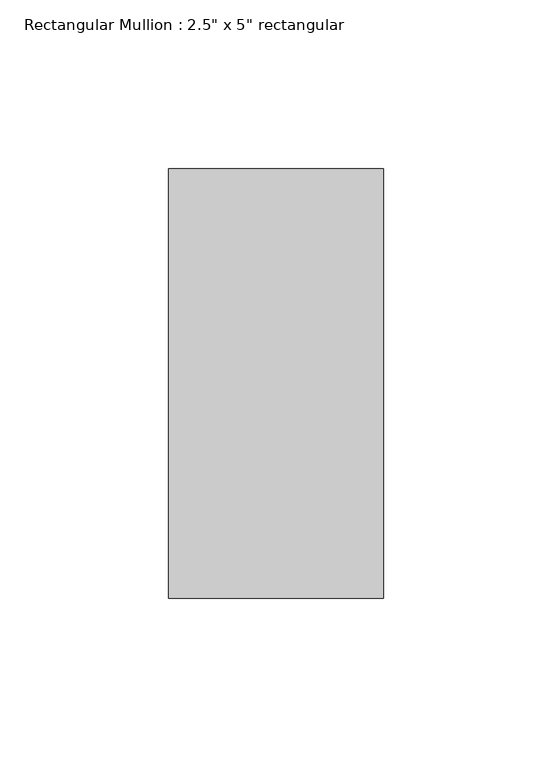
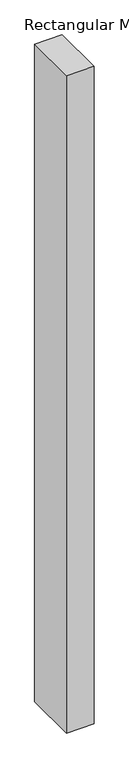
"""IFC4 building model written with IfcOpenShell, lengths in millimetres: member geometry."""

from ifc_helpers import new_model, si_unit, frame, origin, place, context, project, spatial, polyline, outline, extrude, source, transform, mapped, element, save


def member_96e46165(model_context):
    return source(origin(), model_context, "Body", "SweptSolid", [
        extrude(outline(polyline([(31.75, 63.5), (31.75, -63.5), (-31.75, -63.5), (-31.75, 63.5), (31.75, 63.5)])), frame((0.0, 0.0, -1606.2683749), z_axis=(0.0, 0.0, 1.0), x_axis=(1.0, 0.0, 0.0)), (0.0, 0.0, 1.0), 1606.2683749),
    ])


if __name__ == "__main__":
    model = new_model("IFC4")
    model_context = context("Model", 3, world=origin())
    ifc_project = project(units=[si_unit("LENGTHUNIT", "METRE", prefix="MILLI")], contexts=[model_context])
    site = spatial("IfcSite", under=ifc_project)
    building = spatial("IfcBuilding", under=site)
    placement = place(None, origin())
    member_shape = member_96e46165(model_context)
    element("IfcMember", 1, ObjectType="Rectangular Mullion : 2.5\" x 5\" rectangular", at=placement, inside=building, context=model_context, shape_type="MappedRepresentation", body=[
        mapped(member_shape, transform((0.0, 0.0, 0.0), x_axis=(1.0, 0.0, 0.0), y_axis=(0.0, 1.0, 0.0), z_axis=(0.0, 0.0, 1.0))),
    ])
    save(model, "model.ifc")

# Revit data of these elements
# Type "Rectangular Mullion : 2.5\" x 5\" rectangular"
#   built-in parameter 1007304 = 0.416667 (stored number, unit not read)
#   built-in parameter 1007301 = 0.104167 (stored number, unit not read)
#   built-in parameter 1007300 = 0.104167 (stored number, unit not read)
# Element 1 (IfcMember, "Rectangular Mullion : 2.5\" x 5\" rectangular")
#   Materials on its faces: "Aluminum"
# Materials
#   "Aluminum": class "Metal", colour RGB 247 247 247, transparency 0, Description = "Aluminum 6061", Cost = 0
